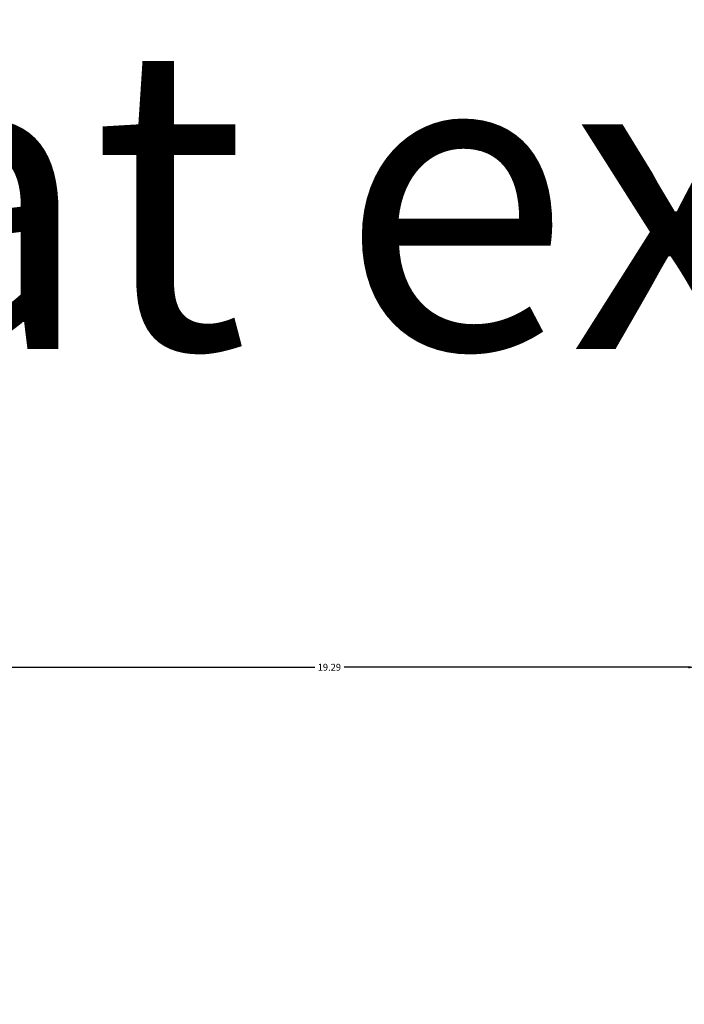
# Model space of a CAD drawing. Units: inches. Extents: x -12 to 334, y -10 to 186.
# Tile 28 of 77: x 88 to 106, y 160 to 186. Entities that reach past the tile are written whole.
import ezdxf

# ---------------------------------------------------------------- set-up
doc = ezdxf.new("R2010")
doc.units = ezdxf.units.IN
doc.header["$MEASUREMENT"] = 0
doc.layers.add('M-ANNO-TEXT', color=3, linetype='Continuous', lineweight=25)
doc.layers.add('M-DIMS', color=2, linetype='Continuous', lineweight=18)
doc.styles.get("Standard").update_dxf_attribs({"font": 'arial.ttf'})
doc.dimstyles.get("Standard").update_dxf_attribs({"dimtxt": 0.18, "dimasz": 0.18, "dimexe": 0.18, "dimexo": 0.0625, "dimgap": 0.09, "dimtad": 0, "dimtih": 1, "dimtoh": 1, "dimdec": 4, "dimzin": 0, "dimdsep": 46, "dimtxsty": 'Standard', "dimcen": 0.09, "dimadec": 0, "dimazin": 0, "dimtfac": 1, "dimtdec": 4, "dimtofl": 0, "dimtmove": 0, "dimatfit": 3, "dimfxl": 1, "dimtolj": 1, "dimtzin": 0, "dimarcsym": 0})

# ---------------------------------------------------------------- blocks, each defined once
blk = doc.blocks.new('*D15')
at = {"layer": 'Defpoints', "color": 0, "transparency": 16777216}
for p in [(106.177, 169.385), (86.888, 109.058), (106.177, 102.896)]:
    blk.add_point(p, dxfattribs=at)
at = {"layer": 'M-DIMS', "color": 0, "lineweight": -2, "transparency": 16777216}
for p, q in [((86.888, 109.121), (86.888, 169.565)), ((87.068, 169.385), (96.147, 169.385)), ((105.997, 169.385), (96.918, 169.385)), ((106.177, 102.958), (106.177, 169.565))]:
    blk.add_line(p, q, dxfattribs=at)
at = {"layer": 'M-DIMS', "color": 0, "transparency": 16777216}
for points in [[(87.068, 169.415), (87.068, 169.355), (86.888, 169.385)], [(105.997, 169.415), (105.997, 169.355), (106.177, 169.385)]]:
    blk.add_solid(points, dxfattribs=at)
at = {"layer": 'M-DIMS', "color": 0, "transparency": 16777216, "insert": (96.532, 169.385), "char_height": 0.18, "attachment_point": 5}
blk.add_mtext('\\A1;19.29', dxfattribs=at)

msp = doc.modelspace()

# ---------------------------------------------------------------- texts
at = {"layer": 'M-ANNO-TEXT', "insert": (70.1252, 185.7805), "char_height": 8, "attachment_point": 1}
msp.add_mtext_dynamic_manual_height_columns('Heat exchanger in a steam boiler', width=205.597506, gutter_width=1, heights=[0], dxfattribs=at)

# ---------------------------------------------------------------- dimensions: what is measured, and where the dimension line sits
at = {"layer": 'M-DIMS'}
dim = msp.add_linear_dim(base=(106.1771, 169.3845), p1=(86.8879, 109.0583), p2=(106.1771, 102.8958), dimstyle='Standard', override={"dimdec": 2, "dimlfac": 1, "dimrnd": 0, "dimzin": 0, "dimdsep": 46, "dimlunit": 2}, dxfattribs=at)
dim.commit()
dim.dimension.update_dxf_attribs({"geometry": '*D15', "text_midpoint": (96.5325, 169.3845)})

doc.saveas('drawing.dxf')
